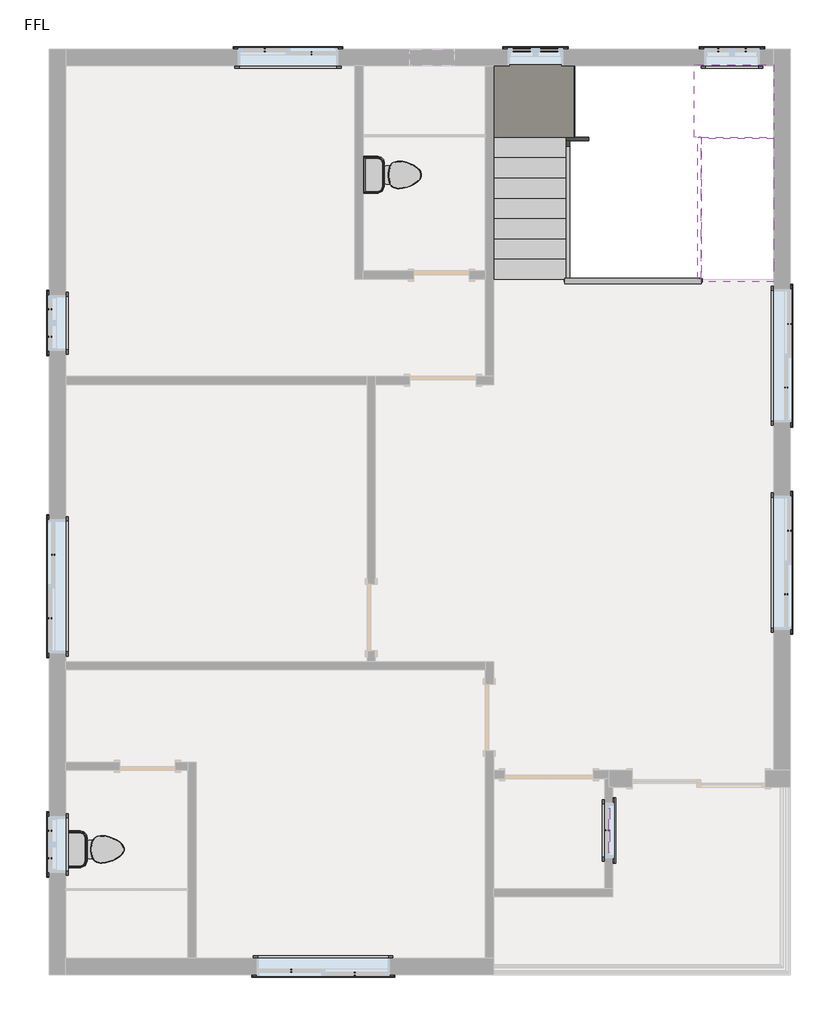
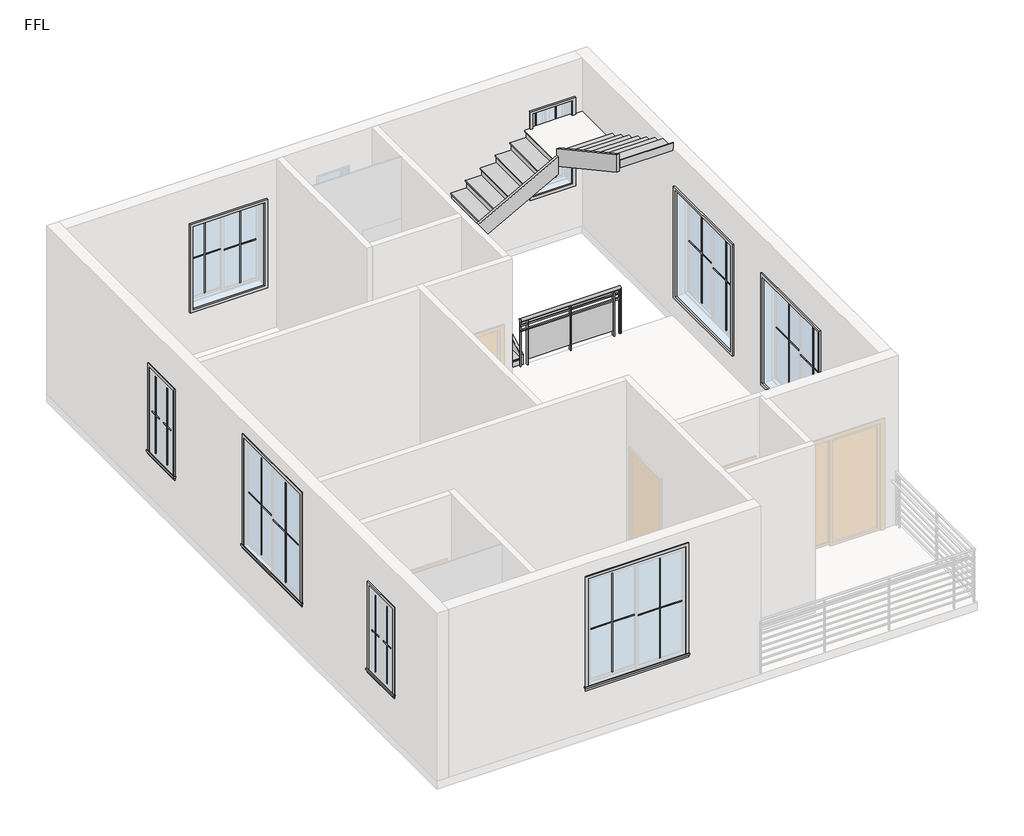
# One storey, part 3 of 3: 40 proxies, 3 members, 3 stair flights, 2 flow terminals, 2 slabs, 1 railing.
"""IFC4 building model written with IfcOpenShell, lengths in millimetres."""

from ifc_helpers import new_model, si_unit, point, frame, origin, place, context, project, spatial, polyline, ellipse_curve, trimmed, outline, extrude, faceted_brep, transform, mapped, element, save
from ifc_brep_helpers import plane_surface, extruded_surface, advanced_brep
from components import muntin_pattern_2x2_muntin_pattern_2x2_bf2b9acc, muntin_pattern_2x2_muntin_pattern_2x2_111b6719, muntin_pattern_2x2_muntin_pattern_2x2_1c12c043, muntin_pattern_2x2_muntin_pattern_2x2_88561ff7, muntin_pattern_2x2_muntin_pattern_2x2_b8ba09c9, trim_window_exterior_flat_with_sill_384ab7b4, trim_window_exterior_flat_with_sill_f3cea81b, trim_window_exterior_flat_with_sill_8633aa7b, trim_window_exterior_flat_with_sill_6cd3ad68, trim_window_interior_flat_picture_frame_e62f86b4, trim_window_interior_flat_picture_frame_717249e1, trim_window_interior_flat_picture_frame_129e3d92, trim_window_interior_flat_picture_frame_840a62db, toilet_domestic_3d_toilet_domestic_3d_ba6479b0, toilet_domestic_3d_toilet_domestic_3d_30431060, non_monolithic_landing_c2e7054d, non_monolithic_landing_4949486c, stair_flight_7d9c97bb, stair_flight_69e76367, stair_flight_2b7c7c02

model = new_model("IFC4")

# Units and contexts
model_context = context("Model", 3, world=origin())
ifc_project = project(units=[si_unit("LENGTHUNIT", "METRE", prefix="MILLI")], contexts=[model_context])

# Site, building, storey
site = spatial("IfcSite", under=ifc_project)
building = spatial("IfcBuilding", under=site)
storey = spatial("IfcBuildingStorey", under=building, Name="FFL", Elevation=3505.2)

# Proxies
placement = place(None, origin())
muntin_pattern_2x2_muntin_pattern_2x2_shape = muntin_pattern_2x2_muntin_pattern_2x2_bf2b9acc(model_context)
element("IfcBuildingElementProxy", 1, Name="Muntin Pattern_2x2 : Muntin Pattern_2x2", ObjectType="Muntin Pattern_2x2 : Muntin Pattern_2x2", at=placement, inside=storey, context=model_context, shape_type="MappedRepresentation", body=[
    mapped(muntin_pattern_2x2_muntin_pattern_2x2_shape, transform((-10595.313469, -269.4121638, 4502.15), x_axis=(-1.0, 0.0, 0.0), y_axis=(0.0, -1.0, 0.0), z_axis=(0.0, 0.0, 1.0))),
])
element("IfcBuildingElementProxy", 2, Name="Muntin Pattern_2x2 : Muntin Pattern_2x2", ObjectType="Muntin Pattern_2x2 : Muntin Pattern_2x2", at=placement, inside=storey, context=model_context, shape_type="MappedRepresentation", body=[
    mapped(muntin_pattern_2x2_muntin_pattern_2x2_shape, transform((-9722.188469, -313.8621638, 4502.15), x_axis=(-1.0, 0.0, 0.0), y_axis=(0.0, -1.0, 0.0), z_axis=(0.0, 0.0, 1.0))),
])
element("IfcBuildingElementProxy", 3, Name="Muntin Pattern_2x2 : Muntin Pattern_2x2", ObjectType="Muntin Pattern_2x2 : Muntin Pattern_2x2", at=placement, inside=storey, context=model_context, shape_type="MappedRepresentation", body=[
    mapped(muntin_pattern_2x2_muntin_pattern_2x2_shape, transform((-13870.3252526, 5453.5252283, 4502.15), x_axis=(0.0, 1.0, 0.0), y_axis=(-1.0, 0.0, 0.0), z_axis=(0.0, 0.0, 1.0))),
])
element("IfcBuildingElementProxy", 4, Name="Muntin Pattern_2x2 : Muntin Pattern_2x2", ObjectType="Muntin Pattern_2x2 : Muntin Pattern_2x2", at=placement, inside=storey, context=model_context, shape_type="MappedRepresentation", body=[
    mapped(muntin_pattern_2x2_muntin_pattern_2x2_shape, transform((-13914.7752526, 4580.4002283, 4502.15), x_axis=(0.0, 1.0, 0.0), y_axis=(-1.0, 0.0, 0.0), z_axis=(0.0, 0.0, 1.0))),
])
element("IfcBuildingElementProxy", 5, Name="Muntin Pattern_2x2 : Muntin Pattern_2x2", ObjectType="Muntin Pattern_2x2 : Muntin Pattern_2x2", at=placement, inside=storey, context=model_context, shape_type="MappedRepresentation", body=[
    mapped(muntin_pattern_2x2_muntin_pattern_2x2_shape, transform((-3789.7007748, 4906.3170268, 4044.95), x_axis=(0.0, -1.0, 0.0), y_axis=(1.0, 0.0, 0.0), z_axis=(0.0, 0.0, 1.0))),
])
element("IfcBuildingElementProxy", 6, Name="Muntin Pattern_2x2 : Muntin Pattern_2x2", ObjectType="Muntin Pattern_2x2 : Muntin Pattern_2x2", at=placement, inside=storey, context=model_context, shape_type="MappedRepresentation", body=[
    mapped(muntin_pattern_2x2_muntin_pattern_2x2_shape, transform((-3745.2507748, 5779.4420268, 4044.95), x_axis=(0.0, -1.0, 0.0), y_axis=(1.0, 0.0, 0.0), z_axis=(0.0, 0.0, 1.0))),
])
element("IfcBuildingElementProxy", 7, Name="Muntin Pattern_2x2 : Muntin Pattern_2x2", ObjectType="Muntin Pattern_2x2 : Muntin Pattern_2x2", at=placement, inside=storey, context=model_context, shape_type="MappedRepresentation", body=[
    mapped(muntin_pattern_2x2_muntin_pattern_2x2_shape, transform((-3789.7007748, 7751.1170268, 4044.95), x_axis=(0.0, -1.0, 0.0), y_axis=(1.0, 0.0, 0.0), z_axis=(0.0, 0.0, 1.0))),
])
element("IfcBuildingElementProxy", 8, Name="Muntin Pattern_2x2 : Muntin Pattern_2x2", ObjectType="Muntin Pattern_2x2 : Muntin Pattern_2x2", at=placement, inside=storey, context=model_context, shape_type="MappedRepresentation", body=[
    mapped(muntin_pattern_2x2_muntin_pattern_2x2_shape, transform((-3745.2507748, 8624.2420268, 4044.95), x_axis=(0.0, -1.0, 0.0), y_axis=(1.0, 0.0, 0.0), z_axis=(0.0, 0.0, 1.0))),
])
muntin_pattern_2x2_muntin_pattern_2x2_2_shape = muntin_pattern_2x2_muntin_pattern_2x2_111b6719(model_context)
element("IfcBuildingElementProxy", 9, Name="Muntin Pattern_2x2 : Muntin Pattern_2x2", ObjectType="Muntin Pattern_2x2 : Muntin Pattern_2x2", at=placement, inside=storey, context=model_context, shape_type="MappedRepresentation", body=[
    mapped(muntin_pattern_2x2_muntin_pattern_2x2_2_shape, transform((-10319.0877526, 12348.0378362, 4502.15), x_axis=(1.0, 0.0, 0.0), y_axis=(0.0, 1.0, 0.0), z_axis=(0.0, 0.0, 1.0))),
])
element("IfcBuildingElementProxy", 10, Name="Muntin Pattern_2x2 : Muntin Pattern_2x2", ObjectType="Muntin Pattern_2x2 : Muntin Pattern_2x2", at=placement, inside=storey, context=model_context, shape_type="MappedRepresentation", body=[
    mapped(muntin_pattern_2x2_muntin_pattern_2x2_2_shape, transform((-10963.6127526, 12392.4878362, 4502.15), x_axis=(1.0, 0.0, 0.0), y_axis=(0.0, 1.0, 0.0), z_axis=(0.0, 0.0, 1.0))),
])
muntin_pattern_2x2_muntin_pattern_2x2_3_shape = muntin_pattern_2x2_muntin_pattern_2x2_1c12c043(model_context)
element("IfcBuildingElementProxy", 11, Name="Muntin Pattern_2x2 : Muntin Pattern_2x2", ObjectType="Muntin Pattern_2x2 : Muntin Pattern_2x2", at=placement, inside=storey, context=model_context, shape_type="MappedRepresentation", body=[
    mapped(muntin_pattern_2x2_muntin_pattern_2x2_3_shape, transform((-13914.7752526, 8447.5503362, 4489.45), x_axis=(0.0, 1.0, 0.0), y_axis=(-1.0, 0.0, 0.0), z_axis=(0.0, 0.0, 1.0))),
])
element("IfcBuildingElementProxy", 12, Name="Muntin Pattern_2x2 : Muntin Pattern_2x2", ObjectType="Muntin Pattern_2x2 : Muntin Pattern_2x2", at=placement, inside=storey, context=model_context, shape_type="MappedRepresentation", body=[
    mapped(muntin_pattern_2x2_muntin_pattern_2x2_3_shape, transform((-13914.7752526, 1278.4003362, 4489.45), x_axis=(0.0, 1.0, 0.0), y_axis=(-1.0, 0.0, 0.0), z_axis=(0.0, 0.0, 1.0))),
])
element("IfcBuildingElementProxy", 13, Name="Muntin Pattern_2x2 : Muntin Pattern_2x2", ObjectType="Muntin Pattern_2x2 : Muntin Pattern_2x2", at=placement, inside=storey, context=model_context, shape_type="MappedRepresentation", body=[
    mapped(muntin_pattern_2x2_muntin_pattern_2x2_3_shape, transform((-7426.6627526, 12392.4878362, 3575.05), x_axis=(1.0, 0.0, 0.0), y_axis=(0.0, 1.0, 0.0), z_axis=(0.0, 0.0, 1.0))),
])
element("IfcBuildingElementProxy", 14, Name="Muntin Pattern_2x2 : Muntin Pattern_2x2", ObjectType="Muntin Pattern_2x2 : Muntin Pattern_2x2", at=placement, inside=storey, context=model_context, shape_type="MappedRepresentation", body=[
    mapped(muntin_pattern_2x2_muntin_pattern_2x2_3_shape, transform((-4724.7382748, 12392.4878362, 4489.45), x_axis=(1.0, 0.0, 0.0), y_axis=(0.0, 1.0, 0.0), z_axis=(0.0, 0.0, 1.0))),
])
muntin_pattern_2x2_muntin_pattern_2x2_4_shape = muntin_pattern_2x2_muntin_pattern_2x2_88561ff7(model_context)
element("IfcBuildingElementProxy", 15, Name="Muntin Pattern_2x2 : Muntin Pattern_2x2", ObjectType="Muntin Pattern_2x2 : Muntin Pattern_2x2", at=placement, inside=storey, context=model_context, shape_type="MappedRepresentation", body=[
    mapped(muntin_pattern_2x2_muntin_pattern_2x2_4_shape, transform((-13914.7752526, 8825.3753362, 4489.45), x_axis=(0.0, -1.0, 0.0), y_axis=(1.0, 0.0, 0.0), z_axis=(0.0, 0.0, 1.0))),
])
element("IfcBuildingElementProxy", 16, Name="Muntin Pattern_2x2 : Muntin Pattern_2x2", ObjectType="Muntin Pattern_2x2 : Muntin Pattern_2x2", at=placement, inside=storey, context=model_context, shape_type="MappedRepresentation", body=[
    mapped(muntin_pattern_2x2_muntin_pattern_2x2_4_shape, transform((-13914.7752526, 1656.2253362, 4489.45), x_axis=(0.0, -1.0, 0.0), y_axis=(1.0, 0.0, 0.0), z_axis=(0.0, 0.0, 1.0))),
])
element("IfcBuildingElementProxy", 17, Name="Muntin Pattern_2x2 : Muntin Pattern_2x2", ObjectType="Muntin Pattern_2x2 : Muntin Pattern_2x2", at=placement, inside=storey, context=model_context, shape_type="MappedRepresentation", body=[
    mapped(muntin_pattern_2x2_muntin_pattern_2x2_4_shape, transform((-7048.8377526, 12392.4878362, 3575.05), x_axis=(-1.0, 0.0, 0.0), y_axis=(0.0, -1.0, 0.0), z_axis=(0.0, 0.0, 1.0))),
])
element("IfcBuildingElementProxy", 18, Name="Muntin Pattern_2x2 : Muntin Pattern_2x2", ObjectType="Muntin Pattern_2x2 : Muntin Pattern_2x2", at=placement, inside=storey, context=model_context, shape_type="MappedRepresentation", body=[
    mapped(muntin_pattern_2x2_muntin_pattern_2x2_4_shape, transform((-4346.9132748, 12392.4878362, 4489.45), x_axis=(-1.0, 0.0, 0.0), y_axis=(0.0, -1.0, 0.0), z_axis=(0.0, 0.0, 1.0))),
])
muntin_pattern_2x2_muntin_pattern_2x2_5_shape = muntin_pattern_2x2_muntin_pattern_2x2_b8ba09c9(model_context)
element("IfcBuildingElementProxy", 19, Name="Muntin Pattern_2x2 : Muntin Pattern_2x2", ObjectType="Muntin Pattern_2x2 : Muntin Pattern_2x2", at=placement, inside=storey, context=model_context, shape_type="MappedRepresentation", body=[
    mapped(muntin_pattern_2x2_muntin_pattern_2x2_5_shape, transform((-6209.0507748, 1659.8795268, 5026.025), x_axis=(0.0, -1.0, 0.0), y_axis=(1.0, 0.0, 0.0), z_axis=(0.0, 0.0, 1.0))),
])
element("IfcBuildingElementProxy", 20, Name="Muntin Pattern_2x2 : Muntin Pattern_2x2", ObjectType="Muntin Pattern_2x2 : Muntin Pattern_2x2", at=placement, inside=storey, context=model_context, shape_type="MappedRepresentation", body=[
    mapped(muntin_pattern_2x2_muntin_pattern_2x2_5_shape, transform((-6253.5007748, 1659.8795268, 4495.8), x_axis=(0.0, -1.0, 0.0), y_axis=(1.0, 0.0, 0.0), z_axis=(0.0, 0.0, 1.0))),
])
trim_window_exterior_flat_with_sill_shape = trim_window_exterior_flat_with_sill_384ab7b4(model_context)
element("IfcBuildingElementProxy", 21, Name="Trim-Window-Exterior-Flat : with Sill", ObjectType="Trim-Window-Exterior-Flat : with Sill", at=placement, inside=storey, context=model_context, shape_type="MappedRepresentation", body=[
    mapped(trim_window_exterior_flat_with_sill_shape, transform((-10158.750969, -323.3871638, 6553.2), x_axis=(1.0, 0.0, 0.0), y_axis=(0.0, 0.0, 1.0), z_axis=(0.0, -1.0, 0.0))),
])
element("IfcBuildingElementProxy", 22, Name="Trim-Window-Exterior-Flat : with Sill", ObjectType="Trim-Window-Exterior-Flat : with Sill", at=placement, inside=storey, context=model_context, shape_type="MappedRepresentation", body=[
    mapped(trim_window_exterior_flat_with_sill_shape, transform((-13924.3002526, 5016.9627283, 6553.2), x_axis=(0.0, -1.0, 0.0), y_axis=(0.0, 0.0, 1.0), z_axis=(-1.0, 0.0, 0.0))),
])
element("IfcBuildingElementProxy", 23, Name="Trim-Window-Exterior-Flat : with Sill", ObjectType="Trim-Window-Exterior-Flat : with Sill", at=placement, inside=storey, context=model_context, shape_type="MappedRepresentation", body=[
    mapped(trim_window_exterior_flat_with_sill_shape, transform((-3735.7257748, 5342.8795268, 6096.0), x_axis=(0.0, 1.0, 0.0), y_axis=(0.0, 0.0, 1.0), z_axis=(1.0, 0.0, 0.0))),
])
element("IfcBuildingElementProxy", 24, Name="Trim-Window-Exterior-Flat : with Sill", ObjectType="Trim-Window-Exterior-Flat : with Sill", at=placement, inside=storey, context=model_context, shape_type="MappedRepresentation", body=[
    mapped(trim_window_exterior_flat_with_sill_shape, transform((-3735.7257748, 8187.6795268, 6096.0), x_axis=(0.0, 1.0, 0.0), y_axis=(0.0, 0.0, 1.0), z_axis=(1.0, 0.0, 0.0))),
])
trim_window_exterior_flat_with_sill_2_shape = trim_window_exterior_flat_with_sill_f3cea81b(model_context)
element("IfcBuildingElementProxy", 25, Name="Trim-Window-Exterior-Flat : with Sill", ObjectType="Trim-Window-Exterior-Flat : with Sill", at=placement, inside=storey, context=model_context, shape_type="MappedRepresentation", body=[
    mapped(trim_window_exterior_flat_with_sill_2_shape, transform((-10641.3502526, 12402.0128362, 6096.0), x_axis=(-1.0, 0.0, 0.0), y_axis=(0.0, 0.0, 1.0), z_axis=(0.0, 1.0, 0.0))),
])
trim_window_exterior_flat_with_sill_3_shape = trim_window_exterior_flat_with_sill_8633aa7b(model_context)
element("IfcBuildingElementProxy", 26, Name="Trim-Window-Exterior-Flat : with Sill", ObjectType="Trim-Window-Exterior-Flat : with Sill", at=placement, inside=storey, context=model_context, shape_type="MappedRepresentation", body=[
    mapped(trim_window_exterior_flat_with_sill_3_shape, transform((-13924.3002526, 8636.4628362, 6096.0), x_axis=(0.0, -1.0, 0.0), y_axis=(0.0, 0.0, 1.0), z_axis=(-1.0, 0.0, 0.0))),
])
element("IfcBuildingElementProxy", 27, Name="Trim-Window-Exterior-Flat : with Sill", ObjectType="Trim-Window-Exterior-Flat : with Sill", at=placement, inside=storey, context=model_context, shape_type="MappedRepresentation", body=[
    mapped(trim_window_exterior_flat_with_sill_3_shape, transform((-13924.3002526, 1467.3128362, 6096.0), x_axis=(0.0, -1.0, 0.0), y_axis=(0.0, 0.0, 1.0), z_axis=(-1.0, 0.0, 0.0))),
])
element("IfcBuildingElementProxy", 28, Name="Trim-Window-Exterior-Flat : with Sill", ObjectType="Trim-Window-Exterior-Flat : with Sill", at=placement, inside=storey, context=model_context, shape_type="MappedRepresentation", body=[
    mapped(trim_window_exterior_flat_with_sill_3_shape, transform((-7237.7502526, 12402.0128362, 5181.6), x_axis=(-1.0, 0.0, 0.0), y_axis=(0.0, 0.0, 1.0), z_axis=(0.0, 1.0, 0.0))),
])
element("IfcBuildingElementProxy", 29, Name="Trim-Window-Exterior-Flat : with Sill", ObjectType="Trim-Window-Exterior-Flat : with Sill", at=placement, inside=storey, context=model_context, shape_type="MappedRepresentation", body=[
    mapped(trim_window_exterior_flat_with_sill_3_shape, transform((-4535.8257748, 12402.0128362, 6096.0), x_axis=(-1.0, 0.0, 0.0), y_axis=(0.0, 0.0, 1.0), z_axis=(0.0, 1.0, 0.0))),
])
trim_window_exterior_flat_with_sill_4_shape = trim_window_exterior_flat_with_sill_6cd3ad68(model_context)
element("IfcBuildingElementProxy", 30, Name="Trim-Window-Exterior-Flat : with Sill", ObjectType="Trim-Window-Exterior-Flat : with Sill", at=placement, inside=storey, context=model_context, shape_type="MappedRepresentation", body=[
    mapped(trim_window_exterior_flat_with_sill_4_shape, transform((-6174.1257748, 1659.8795268, 5588.0), x_axis=(0.0, 1.0, 0.0), y_axis=(0.0, 0.0, 1.0), z_axis=(1.0, 0.0, 0.0))),
])
trim_window_interior_flat_picture_frame_shape = trim_window_interior_flat_picture_frame_e62f86b4(model_context)
element("IfcBuildingElementProxy", 31, Name="Trim-Window-Interior-Flat : Picture Frame", ObjectType="Trim-Window-Interior-Flat : Picture Frame", at=placement, inside=storey, context=model_context, shape_type="MappedRepresentation", body=[
    mapped(trim_window_interior_flat_picture_frame_shape, transform((-10158.750969, -94.7871638, 6553.2), x_axis=(-1.0, 0.0, 0.0), y_axis=(0.0, 0.0, 1.0), z_axis=(0.0, 1.0, 0.0))),
])
element("IfcBuildingElementProxy", 32, Name="Trim-Window-Interior-Flat : Picture Frame", ObjectType="Trim-Window-Interior-Flat : Picture Frame", at=placement, inside=storey, context=model_context, shape_type="MappedRepresentation", body=[
    mapped(trim_window_interior_flat_picture_frame_shape, transform((-13695.7002526, 5016.9627283, 6553.2), x_axis=(0.0, 1.0, 0.0), y_axis=(0.0, 0.0, 1.0), z_axis=(1.0, 0.0, 0.0))),
])
element("IfcBuildingElementProxy", 33, Name="Trim-Window-Interior-Flat : Picture Frame", ObjectType="Trim-Window-Interior-Flat : Picture Frame", at=placement, inside=storey, context=model_context, shape_type="MappedRepresentation", body=[
    mapped(trim_window_interior_flat_picture_frame_shape, transform((-3964.3257748, 5342.8795268, 6096.0), x_axis=(0.0, -1.0, 0.0), y_axis=(0.0, 0.0, 1.0), z_axis=(-1.0, 0.0, 0.0))),
])
element("IfcBuildingElementProxy", 34, Name="Trim-Window-Interior-Flat : Picture Frame", ObjectType="Trim-Window-Interior-Flat : Picture Frame", at=placement, inside=storey, context=model_context, shape_type="MappedRepresentation", body=[
    mapped(trim_window_interior_flat_picture_frame_shape, transform((-3964.3257748, 8187.6795268, 6096.0), x_axis=(0.0, -1.0, 0.0), y_axis=(0.0, 0.0, 1.0), z_axis=(-1.0, 0.0, 0.0))),
])
trim_window_interior_flat_picture_frame_2_shape = trim_window_interior_flat_picture_frame_717249e1(model_context)
element("IfcBuildingElementProxy", 35, Name="Trim-Window-Interior-Flat : Picture Frame", ObjectType="Trim-Window-Interior-Flat : Picture Frame", at=placement, inside=storey, context=model_context, shape_type="MappedRepresentation", body=[
    mapped(trim_window_interior_flat_picture_frame_2_shape, transform((-10641.3502526, 12173.4128362, 6096.0), x_axis=(1.0, 0.0, 0.0), y_axis=(0.0, 0.0, 1.0), z_axis=(0.0, -1.0, 0.0))),
])
trim_window_interior_flat_picture_frame_3_shape = trim_window_interior_flat_picture_frame_129e3d92(model_context)
element("IfcBuildingElementProxy", 36, Name="Trim-Window-Interior-Flat : Picture Frame", ObjectType="Trim-Window-Interior-Flat : Picture Frame", at=placement, inside=storey, context=model_context, shape_type="MappedRepresentation", body=[
    mapped(trim_window_interior_flat_picture_frame_3_shape, transform((-13695.7002526, 8636.4628362, 6096.0), x_axis=(0.0, 1.0, 0.0), y_axis=(0.0, 0.0, 1.0), z_axis=(1.0, 0.0, 0.0))),
])
element("IfcBuildingElementProxy", 37, Name="Trim-Window-Interior-Flat : Picture Frame", ObjectType="Trim-Window-Interior-Flat : Picture Frame", at=placement, inside=storey, context=model_context, shape_type="MappedRepresentation", body=[
    mapped(trim_window_interior_flat_picture_frame_3_shape, transform((-13695.7002526, 1467.3128362, 6096.0), x_axis=(0.0, 1.0, 0.0), y_axis=(0.0, 0.0, 1.0), z_axis=(1.0, 0.0, 0.0))),
])
element("IfcBuildingElementProxy", 38, Name="Trim-Window-Interior-Flat : Picture Frame", ObjectType="Trim-Window-Interior-Flat : Picture Frame", at=placement, inside=storey, context=model_context, shape_type="MappedRepresentation", body=[
    mapped(trim_window_interior_flat_picture_frame_3_shape, transform((-7237.7502526, 12173.4128362, 5181.6), x_axis=(1.0, 0.0, 0.0), y_axis=(0.0, 0.0, 1.0), z_axis=(0.0, -1.0, 0.0))),
])
element("IfcBuildingElementProxy", 39, Name="Trim-Window-Interior-Flat : Picture Frame", ObjectType="Trim-Window-Interior-Flat : Picture Frame", at=placement, inside=storey, context=model_context, shape_type="MappedRepresentation", body=[
    mapped(trim_window_interior_flat_picture_frame_3_shape, transform((-4535.8257748, 12173.4128362, 6096.0), x_axis=(1.0, 0.0, 0.0), y_axis=(0.0, 0.0, 1.0), z_axis=(0.0, -1.0, 0.0))),
])
trim_window_interior_flat_picture_frame_4_shape = trim_window_interior_flat_picture_frame_840a62db(model_context)
element("IfcBuildingElementProxy", 40, Name="Trim-Window-Interior-Flat : Picture Frame", ObjectType="Trim-Window-Interior-Flat : Picture Frame", at=placement, inside=storey, context=model_context, shape_type="MappedRepresentation", body=[
    mapped(trim_window_interior_flat_picture_frame_4_shape, transform((-6288.4257748, 1659.8795268, 5588.0), x_axis=(0.0, -1.0, 0.0), y_axis=(0.0, 0.0, 1.0), z_axis=(-1.0, 0.0, 0.0))),
])

# Flow terminals
toilet_domestic_3d_toilet_domestic_3d_shape = toilet_domestic_3d_toilet_domestic_3d_ba6479b0(model_context)
toilet_domestic_3d_toilet_domestic_3d_2_shape = toilet_domestic_3d_toilet_domestic_3d_30431060(model_context)
element("IfcFlowTerminal", 41, ObjectType="Toilet-Domestic-3D : Toilet-Domestic-3D", at=placement, inside=storey, context=model_context, shape_type="MappedRepresentation", body=[
    mapped(toilet_domestic_3d_toilet_domestic_3d_shape, transform((-13201.0042252, 1399.5295268, 3505.2), x_axis=(0.0, 1.0, 0.0), y_axis=(-1.0, 0.0, 0.0), z_axis=(0.0, 0.0, 1.0))),
    mapped(toilet_domestic_3d_toilet_domestic_3d_2_shape, transform((-13201.0042252, 1399.5295268, 3505.2), x_axis=(0.0, 1.0, 0.0), y_axis=(-1.0, 0.0, 0.0), z_axis=(0.0, 0.0, 1.0))),
])
element("IfcFlowTerminal", 42, ObjectType="Toilet-Domestic-3D : Toilet-Domestic-3D", at=placement, inside=storey, context=model_context, shape_type="MappedRepresentation", body=[
    mapped(toilet_domestic_3d_toilet_domestic_3d_shape, transform((-9111.6048726, 10674.8128362, 3505.2), x_axis=(0.0, 1.0, 0.0), y_axis=(-1.0, 0.0, 0.0), z_axis=(0.0, 0.0, 1.0))),
    mapped(toilet_domestic_3d_toilet_domestic_3d_2_shape, transform((-9111.6048726, 10674.8128362, 3505.2), x_axis=(0.0, 1.0, 0.0), y_axis=(-1.0, 0.0, 0.0), z_axis=(0.0, 0.0, 1.0))),
])

# Members
element("IfcMember", 43, ObjectType="Stringer - 2\" Width", at=placement, inside=storey, context=model_context, shape_type="SweptSolid", body=[
    extrude(outline(polyline([(9239.7128362, 3505.2), (9239.7128362, 3711.9436667), (11144.7128362, 4751.0345758), (11144.7128362, 4403.8406619), (9497.2049561, 3505.2), (9239.7128362, 3505.2)])), frame((-6818.6502526, 0.0, 0.0), z_axis=(1.0, 0.0, 0.0), x_axis=(0.0, 1.0, 0.0)), (0.0, 0.0, 1.0), 50.8),
])
element("IfcMember", 44, ObjectType="Stringer - 2\" Width", at=placement, inside=storey, context=model_context, shape_type="SweptSolid", body=[
    extrude(outline(polyline([(4882.6527576, -6818.6502526), (4535.4588436, -6818.6502526), (5522.5952072, -5008.9002526), (5869.7891212, -5008.9002526), (4882.6527576, -6818.6502526)])), frame((0.0, 11144.7128362, 0.0), z_axis=(0.0, 1.0, 0.0), x_axis=(0.0, 0.0, 1.0)), (0.0, 0.0, 1.0), 50.8),
])
element("IfcMember", 45, ObjectType="Stringer - 2\" Width", at=placement, inside=storey, context=model_context, shape_type="SweptSolid", body=[
    extrude(outline(polyline([(11195.5128362, 5997.9436667), (11195.5128362, 5650.7497528), (9239.7128362, 6717.5497528), (9239.7128362, 7064.7436667), (11195.5128362, 5997.9436667)])), frame((-5008.9002526, 0.0, 0.0), z_axis=(1.0, 0.0, 0.0), x_axis=(0.0, 1.0, 0.0)), (0.0, 0.0, 1.0), 50.8),
])

# Railing
element("IfcRailing", 46, ObjectType="Glass Panel - Bottom Fill", at=placement, inside=storey, context=model_context, shape_type="SolidModel", body=[
    advanced_brep(
    [(-6837.7002526, 9252.4128699, 4419.6), (-6837.7002526, 9176.2128699, 4419.6), (-4958.1002526, 9252.4128699, 4419.6), (-4958.1002526, 9176.2128699, 4419.6)],
    [
        (0, 1, ellipse_curve(frame((-6837.7002526, 9214.3128699, 4419.6), z_axis=(-1.0, 0.0, 0.0), x_axis=(0.0, -1.0, 0.0)), 38.1, 28.575)),
        (1, 0, ellipse_curve(frame((-6837.7002526, 9214.3128699, 4419.6), z_axis=(-1.0, 0.0, 0.0), x_axis=(0.0, -1.0, 0.0)), 38.1, 28.575)),
        (2, 3, ellipse_curve(frame((-4958.1002526, 9214.3128699, 4419.6), z_axis=(1.0, 0.0, 0.0), x_axis=(0.0, -1.0, 0.0)), 38.1, 28.575)),
        (3, 2, ellipse_curve(frame((-4958.1002526, 9214.3128699, 4419.6), z_axis=(1.0, 0.0, 0.0), x_axis=(0.0, -1.0, 0.0)), 38.1, 28.575)),
        (0, 2),
        (3, 1),
    ],
    [
        plane_surface(frame((-6837.7002526, 9214.3128699, 4419.6), z_axis=(-1.0, 0.0, 0.0), x_axis=(0.0, 1.0, 0.0))),
        plane_surface(frame((-4958.1002526, 9214.3128699, 4419.6), z_axis=(1.0, 0.0, 0.0), x_axis=(0.0, 1.0, 0.0))),
        extruded_surface(trimmed(ellipse_curve(frame((-4958.1002526, 9214.3128699, 4419.6), z_axis=(-1.0, 0.0, 0.0), x_axis=(0.0, -1.0, 0.0)), 38.1, 28.575), [point((-4958.1002526, 9252.4128699, 4419.6))], [point((-4958.1002526, 9176.2128699, 4419.6))], True, "CARTESIAN"), (-1879.5999999999995, 0.0, 0.0), 1879.5999999999995),
        extruded_surface(trimmed(ellipse_curve(frame((-4958.1002526, 9214.3128699, 4419.6), z_axis=(-1.0, 0.0, 0.0), x_axis=(0.0, -1.0, 0.0)), 38.1, 28.575), [point((-4958.1002526, 9176.2128699, 4419.6))], [point((-4958.1002526, 9252.4128699, 4419.6))], True, "CARTESIAN"), (-1879.5999999999995, 0.0, 0.0), 1879.5999999999995),
    ],
    [
        (0, [[1, 2]]),
        (1, [[3, 4]]),
        (2, [[-1, 5, -4, 6]]),
        (3, [[-2, -6, -3, -5]]),
    ],
),
    faceted_brep([(-6837.7002526, 9201.6128699, 4330.7), (-6837.7002526, 9227.0128699, 4330.7), (-6837.7002526, 9227.0128699, 4305.3), (-6837.7002526, 9201.6128699, 4305.3), (-4945.4002526, 9201.6128699, 4330.7), (-4970.8002526, 9227.0128699, 4330.7), (-4970.8002526, 9227.0128699, 4305.3), (-4945.4002526, 9201.6128699, 4305.3), (-4945.4002526, 9239.7128362, 4330.7), (-4945.4002526, 9239.7128362, 4305.3), (-4970.8002526, 9239.7128362, 4305.3), (-4970.8002526, 9239.7128362, 4330.7)], [[[0, 1, 2, 3]], [[1, 0, 4, 5]], [[2, 1, 5, 6]], [[3, 2, 6, 7]], [[0, 3, 7, 4]], [[8, 9, 10, 11]], [[5, 4, 8, 11]], [[6, 5, 11, 10]], [[7, 6, 10, 9]], [[4, 7, 9, 8]]]),
    faceted_brep([(-6837.7002526, 9201.6128699, 4229.1), (-6837.7002526, 9227.0128699, 4229.1), (-6837.7002526, 9227.0128699, 4203.7), (-6837.7002526, 9201.6128699, 4203.7), (-4945.4002526, 9201.6128699, 4229.1), (-4970.8002526, 9227.0128699, 4229.1), (-4970.8002526, 9227.0128699, 4203.7), (-4945.4002526, 9201.6128699, 4203.7), (-4945.4002526, 9239.7128362, 4229.1), (-4945.4002526, 9239.7128362, 4203.7), (-4970.8002526, 9239.7128362, 4203.7), (-4970.8002526, 9239.7128362, 4229.1)], [[[0, 1, 2, 3]], [[1, 0, 4, 5]], [[2, 1, 5, 6]], [[3, 2, 6, 7]], [[0, 3, 7, 4]], [[8, 9, 10, 11]], [[5, 4, 8, 11]], [[6, 5, 11, 10]], [[7, 6, 10, 9]], [[4, 7, 9, 8]]]),
    extrude(outline(polyline([(-5091.4502526, 9188.9128699), (-5091.4502526, 9239.7128699), (-5078.7502526, 9239.7128699), (-5078.7502526, 9188.9128699), (-5091.4502526, 9188.9128699)])), frame((0.0, 0.0, 3505.2), z_axis=(0.0, 0.0, 1.0), x_axis=(1.0, 0.0, 0.0)), (0.0, 0.0, 1.0), 885.825),
    extrude(outline(polyline([(-5897.9002526, 9220.848027), (-5085.1002526, 9220.848027), (-5085.1002526, 9214.498027), (-5897.9002526, 9214.498027), (-5897.9002526, 9220.848027)])), frame((0.0, 0.0, 3606.8), z_axis=(0.0, 0.0, 1.0), x_axis=(1.0, 0.0, 0.0)), (0.0, 0.0, 1.0), 596.9),
    extrude(outline(polyline([(-5904.2502526, 9188.9128699), (-5904.2502526, 9239.7128699), (-5891.5502526, 9239.7128699), (-5891.5502526, 9188.9128699), (-5904.2502526, 9188.9128699)])), frame((0.0, 0.0, 3505.2), z_axis=(0.0, 0.0, 1.0), x_axis=(1.0, 0.0, 0.0)), (0.0, 0.0, 1.0), 885.825),
    extrude(outline(polyline([(-6710.7002526, 9220.848027), (-5897.9002526, 9220.848027), (-5897.9002526, 9214.498027), (-6710.7002526, 9214.498027), (-6710.7002526, 9220.848027)])), frame((0.0, 0.0, 3606.8), z_axis=(0.0, 0.0, 1.0), x_axis=(1.0, 0.0, 0.0)), (0.0, 0.0, 1.0), 596.9),
    extrude(outline(polyline([(-6717.0502526, 9188.9128699), (-6717.0502526, 9239.7128699), (-6704.3502526, 9239.7128699), (-6704.3502526, 9188.9128699), (-6717.0502526, 9188.9128699)])), frame((0.0, 0.0, 3505.2), z_axis=(0.0, 0.0, 1.0), x_axis=(1.0, 0.0, 0.0)), (0.0, 0.0, 1.0), 885.825),
    extrude(outline(polyline([(-4967.6252526, 9204.7878699), (-4967.6252526, 9223.8378699), (-4948.5752526, 9223.8378699), (-4948.5752526, 9204.7878699), (-4967.6252526, 9204.7878699)])), frame((0.0, 0.0, 3505.2), z_axis=(0.0, 0.0, 1.0), x_axis=(1.0, 0.0, 0.0)), (0.0, 0.0, 1.0), 885.825),
    extrude(outline(polyline([(-4948.5752526, 9227.0128362), (-4967.6252526, 9227.0128362), (-4967.6252526, 9246.0628362), (-4948.5752526, 9246.0628362), (-4948.5752526, 9227.0128362)])), frame((0.0, 0.0, 3505.2), z_axis=(0.0, 0.0, 1.0), x_axis=(1.0, 0.0, 0.0)), (0.0, 0.0, 1.0), 885.825),
    extrude(outline(polyline([(-6844.0502526, 9204.7878699), (-6844.0502526, 9223.8378699), (-6825.0002526, 9223.8378699), (-6825.0002526, 9204.7878699), (-6844.0502526, 9204.7878699)])), frame((0.0, 0.0, 3505.2), z_axis=(0.0, 0.0, 1.0), x_axis=(1.0, 0.0, 0.0)), (0.0, 0.0, 1.0), 885.825),
])

# Slabs
non_monolithic_landing_shape = non_monolithic_landing_c2e7054d(model_context)
element("IfcSlab", 47, ObjectType="Non-Monolithic Landing", at=placement, inside=storey, context=model_context, shape_type="MappedRepresentation", body=[
    mapped(non_monolithic_landing_shape, transform((0.0, 0.0, 0.0), x_axis=(1.0, 0.0, 0.0), y_axis=(0.0, 1.0, 0.0), z_axis=(0.0, 0.0, 1.0))),
])
non_monolithic_landing_2_shape = non_monolithic_landing_4949486c(model_context)
element("IfcSlab", 48, ObjectType="Non-Monolithic Landing", at=placement, inside=storey, context=model_context, shape_type="MappedRepresentation", body=[
    mapped(non_monolithic_landing_2_shape, transform((0.0, 0.0, 0.0), x_axis=(1.0, 0.0, 0.0), y_axis=(0.0, 1.0, 0.0), z_axis=(0.0, 0.0, 1.0))),
])

# Stair flights
stair_flight_shape = stair_flight_7d9c97bb(model_context)
element("IfcStairFlight", 49, ObjectType="2\" Tread 1\" Nosing 1/4\" Riser", at=placement, inside=storey, context=model_context, shape_type="MappedRepresentation", body=[
    mapped(stair_flight_shape, transform((0.0, 0.0, 0.0), x_axis=(1.0, 0.0, 0.0), y_axis=(0.0, 1.0, 0.0), z_axis=(0.0, 0.0, 1.0))),
])
stair_flight_2_shape = stair_flight_69e76367(model_context)
element("IfcStairFlight", 50, ObjectType="2\" Tread 1\" Nosing 1/4\" Riser", at=placement, inside=storey, context=model_context, shape_type="MappedRepresentation", body=[
    mapped(stair_flight_2_shape, transform((0.0, 0.0, 0.0), x_axis=(1.0, 0.0, 0.0), y_axis=(0.0, 1.0, 0.0), z_axis=(0.0, 0.0, 1.0))),
])
stair_flight_3_shape = stair_flight_2b7c7c02(model_context)
element("IfcStairFlight", 51, ObjectType="2\" Tread 1\" Nosing 1/4\" Riser", at=placement, inside=storey, context=model_context, shape_type="MappedRepresentation", body=[
    mapped(stair_flight_3_shape, transform((0.0, 0.0, 0.0), x_axis=(1.0, 0.0, 0.0), y_axis=(0.0, 1.0, 0.0), z_axis=(0.0, 0.0, 1.0))),
])

save(model, "model.ifc")

# Revit data of these elements
# Type "Muntin Pattern_2x2 : Muntin Pattern_2x2"
#   Width [instance default] = 4' - 0"
#   Thickness = 0' - 0 1/2"
#   Height [instance default] = 4' - 0"
#   Distance = 0' - 0 3/4"
#   Interior Material [instance default] = none
#   Exterior Material [instance default] = none
#   Default Elevation = 0
# Type "Trim-Window-Exterior-Flat : with Sill"
#   Trim Width = 0' - 2 1/4"
#   Trim Thickness_Picture Frame = 0' - 1 1/4"
#   Trim Thickness_with Sill = 0' - 0 3/4"
#   Sill Thickness = 0' - 1 1/4"
#   Opening Width [instance default] = 2' - 0"
#   Opening Height [instance default] = 3' - 0"
#   Default Elevation = 4' - 0"
#   Sill = yes
#   Picture Frame = no
#   Trim Material [instance default] = none
# Type "Trim-Window-Interior-Flat : Picture Frame"
#   Trim Thickness_Picture Frame = 0' - 1 1/4"
#   Trim Width = 0' - 2 1/4"
#   Trim Thickness_with Sill = 0' - 0 3/4"
#   Sill Thickness = 0' - 1 1/4"
#   Opening Width [instance default] = 2' - 0"
#   Opening Height [instance default] = 3' - 0"
#   Default Elevation = 4' - 0"
#   Sill = no
#   Picture Frame = yes
#   Trim Material [instance default] = none
# Type "Toilet-Domestic-3D : Toilet-Domestic-3D"
#   Assembly Code = "D2010110"
#   Toilet - Bowl/Basin Material = Porcelain, Linen
#   Toilet - Seat Material = Laminate, Linen, Matte
#   Default Elevation = 0
# Type "Glass Panel - Bottom Fill"
#   Assembly Code = "C2010400"
#   built-in parameter 1008612 = 0.0416667 (stored number, unit not read)
#   built-in parameter 1008611 = 0.0416667 (stored number, unit not read)
#   built-in parameter 1008609 = 0.333333 (stored number, unit not read)
#   built-in parameter 1008604 = 0.166667 (stored number, unit not read)
#   built-in parameter 1008603 = 0.166667 (stored number, unit not read)
#   Railing Height = 3' - 0"
#   built-in parameter 1008630 = 2
#   built-in parameter 1008610 = 2
#   built-in parameter 1008618 = Baluster - Square : 3/4"
# Elements 1, 2, 3, 4, 5, 6, 7, 8 (IfcBuildingElementProxy, "Muntin Pattern_2x2 : Muntin Pattern_2x2")
#   Width = 2' - 8 5/8"
#   Height = 6' - 6 1/4"
#   Interior Material = Wood - Stained
#   Exterior Material = Clad - White
#   Phase Created = New Construction
#   Materials on its faces: "Clad - White", "Wood - Stained"
# Elements 9, 10 (IfcBuildingElementProxy, "Muntin Pattern_2x2 : Muntin Pattern_2x2")
#   Width = 1' - 11 5/8"
#   Height = 5' - 0 1/4"
#   Interior Material = Wood - Stained
#   Exterior Material = Clad - White
#   Phase Created = New Construction
#   Materials on its faces: "Clad - White", "Wood - Stained"
# Elements 11, 12, 13, 14, 15, 16, 17, 18 (IfcBuildingElementProxy, "Muntin Pattern_2x2 : Muntin Pattern_2x2")
#   Width = 0' - 9 5/8"
#   Height = 5' - 0 1/2"
#   Interior Material = Wood - Stained
#   Exterior Material = Clad - White
#   Phase Created = New Construction
#   Materials on its faces: "Clad - White", "Wood - Stained"
# Elements 19, 20 (IfcBuildingElementProxy, "Muntin Pattern_2x2 : Muntin Pattern_2x2")
#   Width = 2' - 0"
#   Height = 1' - 7 1/8"
#   Interior Material = Wood - Stained
#   Exterior Material = Clad - White
#   Phase Created = New Construction
#   Materials on its faces: "Clad - White", "Wood - Stained"
# Elements 21, 22, 23, 24 (IfcBuildingElementProxy, "Trim-Window-Exterior-Flat : with Sill")
#   Opening Width = 6' - 0"
#   Opening Height = 7' - 0"
#   Trim Material = Clad - White
#   Phase Created = New Construction
#   Materials on its faces: "Clad - White"
# Element 25 (IfcBuildingElementProxy, "Trim-Window-Exterior-Flat : with Sill")
#   Opening Width = 4' - 6"
#   Opening Height = 5' - 6"
#   Trim Material = Clad - White
#   Phase Created = New Construction
#   Materials on its faces: "Clad - White"
# Elements 26, 27, 28, 29 (IfcBuildingElementProxy, "Trim-Window-Exterior-Flat : with Sill")
#   Opening Width = 2' - 6"
#   Opening Height = 5' - 6"
#   Trim Material = Clad - White
#   Phase Created = New Construction
#   Materials on its faces: "Clad - White"
# Element 30 (IfcBuildingElementProxy, "Trim-Window-Exterior-Flat : with Sill")
#   Opening Width = 2' - 6"
#   Opening Height = 3' - 10"
#   Trim Material = Clad - White
#   Phase Created = New Construction
#   Materials on its faces: "Clad - White"
# Elements 31, 32, 33, 34 (IfcBuildingElementProxy, "Trim-Window-Interior-Flat : Picture Frame")
#   Opening Width = 6' - 0"
#   Opening Height = 7' - 0"
#   Trim Material = Wood - Stained
#   Phase Created = New Construction
#   Materials on its faces: "Wood - Stained"
# Element 35 (IfcBuildingElementProxy, "Trim-Window-Interior-Flat : Picture Frame")
#   Opening Width = 4' - 6"
#   Opening Height = 5' - 6"
#   Trim Material = Wood - Stained
#   Phase Created = New Construction
#   Materials on its faces: "Wood - Stained"
# Elements 36, 37, 38, 39 (IfcBuildingElementProxy, "Trim-Window-Interior-Flat : Picture Frame")
#   Opening Width = 2' - 6"
#   Opening Height = 5' - 6"
#   Trim Material = Wood - Stained
#   Phase Created = New Construction
#   Materials on its faces: "Wood - Stained"
# Element 40 (IfcBuildingElementProxy, "Trim-Window-Interior-Flat : Picture Frame")
#   Opening Width = 2' - 6"
#   Opening Height = 3' - 10"
#   Trim Material = Wood - Stained
#   Phase Created = New Construction
#   Materials on its faces: "Wood - Stained"
# Element 41 (IfcFlowTerminal, "Toilet-Domestic-3D : Toilet-Domestic-3D")
#   Mark = "4"
#   Phase Created = New Construction
#   Materials on its faces: "Porcelain, Linen", "Laminate, Linen, Matte"
# Element 42 (IfcFlowTerminal, "Toilet-Domestic-3D : Toilet-Domestic-3D")
#   Mark = "5"
#   Phase Created = New Construction
#   Materials on its faces: "Porcelain, Linen", "Laminate, Linen, Matte"
# Elements 43, 44, 45 (IfcMember, "Stringer - 2\" Width")
#   Phase Created = New Construction
# Element 46 (IfcRailing, "Glass Panel - Bottom Fill")
#   Phase Created = New Construction
#   Materials on its faces: "Glass"
# Elements 47, 48 (IfcSlab, "Non-Monolithic Landing")
#   Phase Created = New Construction
# Elements 49, 50, 51 (IfcStairFlight, "2\" Tread 1\" Nosing 1/4\" Riser")
#   Phase Created = New Construction
# Materials
#   "Porcelain, Linen": class "Ceramic", colour RGB 249 239 230, transparency 0, Description = "Porcelain, linen", Cost = 0
#   "Laminate, Linen, Matte": class "Plastic", colour RGB 249 239 230, transparency 0, Description = "Plastic Laminate - Linen, Matte", Cost = 0
#   "Clad - White": class "Wood", colour RGB 242 242 238, transparency 0, Cost = 0
#   "Wood - Stained": class "Wood", colour RGB 224 178 126, transparency 0, Cost = 0
#   "Glass": class "Glass", colour RGB 0 128 192, transparency 0.75, Description = "Soda Lime Glass", Cost = 0
